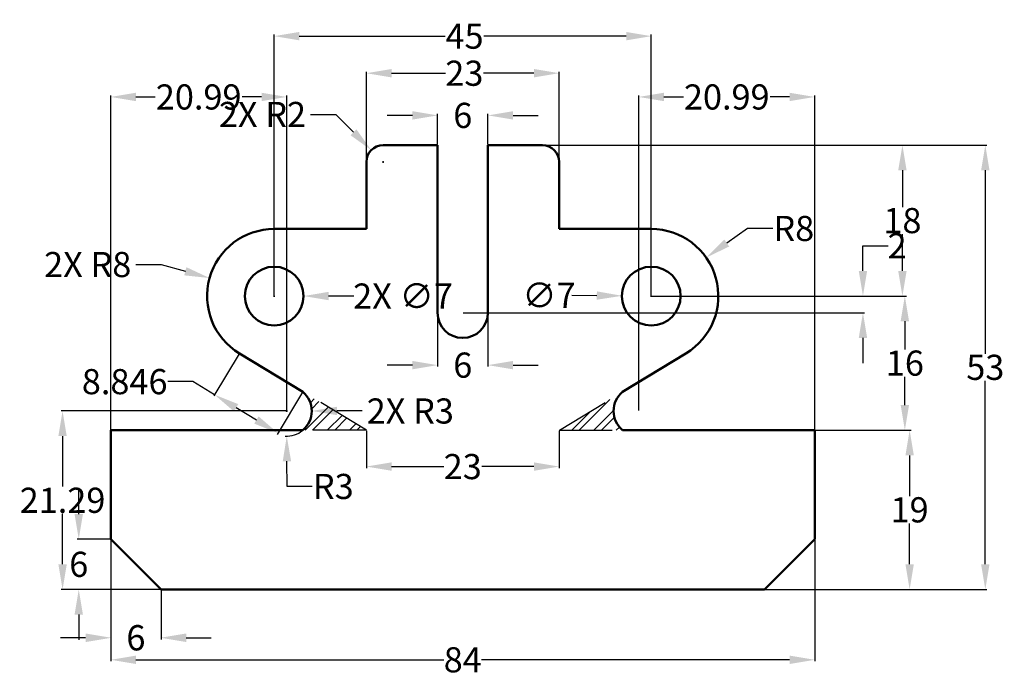
# Model space of a CAD drawing. Units: inches. Extents: x 2 to 120, y -4 to 75.
import ezdxf

# ---------------------------------------------------------------- set-up
doc = ezdxf.new("R2010")
doc.units = ezdxf.units.IN
doc.header["$MEASUREMENT"] = 0
doc.linetypes.add('HIDDEN', pattern=[9.525, 6.35, -3.175])
for name, color, linetype, lineweight in [('M-DIMS', 2, 'Continuous', 25), ('M-HATC', 8, 'Continuous', 18), ('M-HIDN', 8, 'HIDDEN', 25), ('M-OUTL', 7, 'Continuous', 50)]:
    doc.layers.add(name, color=color, linetype=linetype, lineweight=lineweight)
doc.styles.get("Standard").update_dxf_attribs({"font": 'arial.ttf'})
doc.dimstyles.get("Standard").update_dxf_attribs({"dimtxt": 3, "dimasz": 3, "dimexe": 0.18, "dimexo": 0.0625, "dimgap": 0.09, "dimtad": 0, "dimtih": 1, "dimtoh": 1, "dimdec": 4, "dimdsep": 46, "dimtxsty": 'Standard', "dimcen": 0.09, "dimadec": 0, "dimazin": 0, "dimtfac": 1, "dimtdec": 4, "dimtofl": 0, "dimtmove": 0, "dimatfit": 3, "dimfxl": 1, "dimtolj": 1, "dimtzin": 0, "dimarcsym": 0})

# ---------------------------------------------------------------- blocks, each defined once
blk = doc.blocks.new('*D1')
at = {"layer": 'Defpoints', "color": 0, "transparency": 16777216}
for p in [(43.51, 25.59), (66.51, 25.59), (66.51, 21.25)]:
    blk.add_point(p, dxfattribs=at)
at = {"layer": 'M-DIMS', "color": 0, "lineweight": -2, "transparency": 16777216}
for p, q in [((43.51, 25.53), (43.51, 21.07)), ((66.51, 25.53), (66.51, 21.07)), ((46.51, 21.25), (52.74, 21.25)), ((63.51, 21.25), (57.27, 21.25))]:
    blk.add_line(p, q, dxfattribs=at)
at = {"layer": 'M-DIMS', "color": 0, "transparency": 16777216}
for points in [[(46.51, 21.75), (46.51, 20.75), (43.51, 21.25)], [(63.51, 21.75), (63.51, 20.75), (66.51, 21.25)]]:
    blk.add_solid(points, dxfattribs=at)
at = {"layer": 'M-DIMS', "color": 0, "transparency": 16777216, "insert": (55.01, 21.25), "char_height": 3, "attachment_point": 5}
blk.add_mtext('\\A1;23', dxfattribs=at)
blk = doc.blocks.new('*D2')
at = {"layer": 'Defpoints', "color": 0, "transparency": 16777216}
for p in [(13.01, 12.59), (97.01, 12.59), (97.01, -1.8)]:
    blk.add_point(p, dxfattribs=at)
at = {"layer": 'M-DIMS', "color": 0, "lineweight": -2, "transparency": 16777216}
for p, q in [((13.01, 12.53), (13.01, -1.98)), ((97.01, 12.53), (97.01, -1.98)), ((16.01, -1.8), (52.77, -1.8)), ((94.01, -1.8), (57.24, -1.8))]:
    blk.add_line(p, q, dxfattribs=at)
at = {"layer": 'M-DIMS', "color": 0, "transparency": 16777216}
for points in [[(16.01, -1.3), (16.01, -2.3), (13.01, -1.8)], [(94.01, -1.3), (94.01, -2.3), (97.01, -1.8)]]:
    blk.add_solid(points, dxfattribs=at)
at = {"layer": 'M-DIMS', "color": 0, "transparency": 16777216, "insert": (55.01, -1.8), "char_height": 3, "attachment_point": 5}
blk.add_mtext('\\A1;84', dxfattribs=at)
blk = doc.blocks.new('*D3')
at = {"layer": 'Defpoints', "color": 0, "transparency": 16777216}
for p in [(13.01, 12.59), (9.19, 6.59), (19.01, 6.59)]:
    blk.add_point(p, dxfattribs=at)
at = {"layer": 'M-DIMS', "color": 0, "lineweight": -2, "transparency": 16777216}
for p, q in [((9.19, 15.59), (9.19, 18.59)), ((12.94, 12.59), (9.01, 12.59)), ((18.94, 6.59), (9.01, 6.59)), ((9.19, 3.59), (9.19, 0.59))]:
    blk.add_line(p, q, dxfattribs=at)
at = {"layer": 'M-DIMS', "color": 0, "transparency": 16777216}
for points in [[(8.69, 15.59), (9.69, 15.59), (9.19, 12.59)], [(8.69, 3.59), (9.69, 3.59), (9.19, 6.59)]]:
    blk.add_solid(points, dxfattribs=at)
at = {"layer": 'M-DIMS', "color": 0, "transparency": 16777216, "insert": (9.19, 9.59), "char_height": 3, "attachment_point": 5}
blk.add_mtext('\\A1;6', dxfattribs=at)
blk = doc.blocks.new('*D4')
at = {"layer": 'Defpoints', "color": 0, "transparency": 16777216}
for p in [(13.01, 12.59), (19.01, 6.59), (19.01, 0.82)]:
    blk.add_point(p, dxfattribs=at)
at = {"layer": 'M-DIMS', "color": 0, "lineweight": -2, "transparency": 16777216}
for p, q in [((13.01, 12.53), (13.01, 0.64)), ((19.01, 6.53), (19.01, 0.64)), ((10.01, 0.82), (7.01, 0.82)), ((22.01, 0.82), (25.01, 0.82))]:
    blk.add_line(p, q, dxfattribs=at)
at = {"layer": 'M-DIMS', "color": 0, "transparency": 16777216}
for points in [[(10.01, 1.32), (10.01, 0.32), (13.01, 0.82)], [(22.01, 1.32), (22.01, 0.32), (19.01, 0.82)]]:
    blk.add_solid(points, dxfattribs=at)
at = {"layer": 'M-DIMS', "color": 0, "transparency": 16777216, "insert": (16.01, 0.82), "char_height": 3, "attachment_point": 5}
blk.add_mtext('\\A1;6', dxfattribs=at)
blk = doc.blocks.new('*D5')
at = {"layer": 'Defpoints', "color": 0, "transparency": 16777216}
for p in [(52.01, 59.59), (58.01, 59.59), (58.01, 33.35)]:
    blk.add_point(p, dxfattribs=at)
at = {"layer": 'M-DIMS', "color": 0, "lineweight": -2, "transparency": 16777216}
for p, q in [((52.01, 59.53), (52.01, 33.17)), ((58.01, 59.53), (58.01, 33.17)), ((49.01, 33.35), (46.01, 33.35)), ((61.01, 33.35), (64.01, 33.35))]:
    blk.add_line(p, q, dxfattribs=at)
at = {"layer": 'M-DIMS', "color": 0, "transparency": 16777216}
for points in [[(49.01, 33.85), (49.01, 32.85), (52.01, 33.35)], [(61.01, 33.85), (61.01, 32.85), (58.01, 33.35)]]:
    blk.add_solid(points, dxfattribs=at)
at = {"layer": 'M-DIMS', "color": 0, "transparency": 16777216, "insert": (55.01, 33.35), "char_height": 3, "attachment_point": 5}
blk.add_mtext('\\A1;6', dxfattribs=at)
blk = doc.blocks.new('*D6')
at = {"layer": 'Defpoints', "color": 0, "transparency": 16777216}
for p in [(77.51, 72.59), (32.51, 41.59), (77.51, 41.59)]:
    blk.add_point(p, dxfattribs=at)
at = {"layer": 'M-DIMS', "color": 0, "lineweight": -2, "transparency": 16777216}
for p, q in [((32.51, 41.65), (32.51, 72.77)), ((35.51, 72.59), (52.91, 72.59)), ((74.51, 72.59), (57.53, 72.59)), ((77.51, 41.65), (77.51, 72.77))]:
    blk.add_line(p, q, dxfattribs=at)
at = {"layer": 'M-DIMS', "color": 0, "transparency": 16777216}
for points in [[(35.51, 73.09), (35.51, 72.09), (32.51, 72.59)], [(74.51, 73.09), (74.51, 72.09), (77.51, 72.59)]]:
    blk.add_solid(points, dxfattribs=at)
at = {"layer": 'M-DIMS', "color": 0, "transparency": 16777216, "insert": (55.22, 72.59), "char_height": 3, "attachment_point": 5}
blk.add_mtext('\\A1;45', dxfattribs=at)
blk = doc.blocks.new('*D7')
at = {"layer": 'Defpoints', "color": 0, "transparency": 16777216}
for p in [(97.01, 25.59), (108.33, 25.59), (91.01, 6.59)]:
    blk.add_point(p, dxfattribs=at)
at = {"layer": 'M-DIMS', "color": 0, "lineweight": -2, "transparency": 16777216}
for p, q in [((97.07, 25.59), (108.51, 25.59)), ((108.33, 22.59), (108.33, 17.71)), ((108.33, 9.59), (108.33, 14.47)), ((91.07, 6.59), (108.51, 6.59))]:
    blk.add_line(p, q, dxfattribs=at)
at = {"layer": 'M-DIMS', "color": 0, "transparency": 16777216}
for points in [[(107.83, 22.59), (108.83, 22.59), (108.33, 25.59)], [(107.83, 9.59), (108.83, 9.59), (108.33, 6.59)]]:
    blk.add_solid(points, dxfattribs=at)
at = {"layer": 'M-DIMS', "color": 0, "transparency": 16777216, "insert": (108.33, 16.09), "char_height": 3, "attachment_point": 5}
blk.add_mtext('\\A1;19', dxfattribs=at)
blk = doc.blocks.new('*D8')
at = {"layer": 'Defpoints', "color": 0, "transparency": 16777216}
for p in [(58.01, 63.14), (52.01, 59.59), (58.01, 59.59)]:
    blk.add_point(p, dxfattribs=at)
at = {"layer": 'M-DIMS', "color": 0, "lineweight": -2, "transparency": 16777216}
for p, q in [((49.01, 63.14), (46.01, 63.14)), ((52.01, 59.65), (52.01, 63.32)), ((58.01, 59.65), (58.01, 63.32)), ((61.01, 63.14), (64.01, 63.14))]:
    blk.add_line(p, q, dxfattribs=at)
at = {"layer": 'M-DIMS', "color": 0, "transparency": 16777216}
for points in [[(49.01, 63.64), (49.01, 62.64), (52.01, 63.14)], [(61.01, 63.64), (61.01, 62.64), (58.01, 63.14)]]:
    blk.add_solid(points, dxfattribs=at)
at = {"layer": 'M-DIMS', "color": 0, "transparency": 16777216, "insert": (55.01, 63.14), "char_height": 3, "attachment_point": 5}
blk.add_mtext('\\A1;6', dxfattribs=at)
blk = doc.blocks.new('*D9')
at = {"layer": 'Defpoints', "color": 0, "transparency": 16777216}
for p in [(77.51, 41.59), (97.01, 25.59), (107.76, 25.59)]:
    blk.add_point(p, dxfattribs=at)
at = {"layer": 'M-DIMS', "color": 0, "lineweight": -2, "transparency": 16777216}
for p, q in [((77.57, 41.59), (107.94, 41.59)), ((107.76, 38.59), (107.76, 35.21)), ((107.76, 28.59), (107.76, 31.97)), ((97.07, 25.59), (107.94, 25.59))]:
    blk.add_line(p, q, dxfattribs=at)
at = {"layer": 'M-DIMS', "color": 0, "transparency": 16777216}
for points in [[(107.26, 38.59), (108.26, 38.59), (107.76, 41.59)], [(107.26, 28.59), (108.26, 28.59), (107.76, 25.59)]]:
    blk.add_solid(points, dxfattribs=at)
at = {"layer": 'M-DIMS', "color": 0, "transparency": 16777216, "insert": (107.76, 33.59), "char_height": 3, "attachment_point": 5}
blk.add_mtext('\\A1;16', dxfattribs=at)
blk = doc.blocks.new('*D10')
at = {"layer": 'Defpoints', "color": 0, "transparency": 16777216}
for p in [(64.51, 59.59), (107.47, 59.59), (77.51, 41.59)]:
    blk.add_point(p, dxfattribs=at)
at = {"layer": 'M-DIMS', "color": 0, "lineweight": -2, "transparency": 16777216}
for p, q in [((64.57, 59.59), (107.65, 59.59)), ((107.47, 56.59), (107.47, 52.21)), ((107.47, 44.59), (107.47, 48.97)), ((77.57, 41.59), (107.65, 41.59))]:
    blk.add_line(p, q, dxfattribs=at)
at = {"layer": 'M-DIMS', "color": 0, "transparency": 16777216}
for points in [[(106.97, 56.59), (107.97, 56.59), (107.47, 59.59)], [(106.97, 44.59), (107.97, 44.59), (107.47, 41.59)]]:
    blk.add_solid(points, dxfattribs=at)
at = {"layer": 'M-DIMS', "color": 0, "transparency": 16777216, "insert": (107.47, 50.59), "char_height": 3, "attachment_point": 5}
blk.add_mtext('\\A1;18', dxfattribs=at)
blk = doc.blocks.new('*D11')
at = {"layer": 'Defpoints', "color": 0, "transparency": 16777216}
for p in [(61.26, 59.59), (61.26, 6.59), (117.36, 6.59)]:
    blk.add_point(p, dxfattribs=at)
at = {"layer": 'M-DIMS', "color": 0, "lineweight": -2, "transparency": 16777216}
for p, q in [((61.32, 59.59), (117.54, 59.59)), ((117.36, 56.59), (117.36, 34.71)), ((117.36, 9.59), (117.36, 31.47)), ((61.32, 6.59), (117.54, 6.59))]:
    blk.add_line(p, q, dxfattribs=at)
at = {"layer": 'M-DIMS', "color": 0, "transparency": 16777216}
for points in [[(116.86, 56.59), (117.86, 56.59), (117.36, 59.59)], [(116.86, 9.59), (117.86, 9.59), (117.36, 6.59)]]:
    blk.add_solid(points, dxfattribs=at)
at = {"layer": 'M-DIMS', "color": 0, "transparency": 16777216, "insert": (117.36, 33.09), "char_height": 3, "attachment_point": 5}
blk.add_mtext('\\A1;53', dxfattribs=at)
blk = doc.blocks.new('*D12')
at = {"layer": 'Defpoints', "color": 0, "transparency": 16777216}
for p in [(74.01, 41.62), (81.01, 41.56)]:
    blk.add_point(p, dxfattribs=at)
at = {"layer": 'M-DIMS', "color": 0, "lineweight": -2, "transparency": 16777216}
for p, q in [((68.01, 41.68), (71.01, 41.65)), ((77.42, 41.59), (77.6, 41.59)), ((77.51, 41.5), (77.51, 41.68))]:
    blk.add_line(p, q, dxfattribs=at)
at = {"layer": 'M-DIMS', "color": 0, "transparency": 16777216}
blk.add_solid([(71.01, 42.15), (71, 41.15), (74.01, 41.62)], dxfattribs=at)
at = {"layer": 'M-DIMS', "color": 0, "transparency": 16777216, "insert": (65.3, 41.68), "char_height": 3, "attachment_point": 5}
blk.add_mtext('\\A1;∅7', dxfattribs=at)
blk = doc.blocks.new('*D13')
at = {"layer": 'Defpoints', "color": 0, "transparency": 16777216}
for p in [(34, 27.88), (34.01, 24.88)]:
    blk.add_point(p, dxfattribs=at)
at = {"layer": 'M-DIMS', "color": 0, "lineweight": -2, "transparency": 16777216}
for p, q in [((33.91, 27.88), (34.09, 27.88)), ((34, 27.79), (34, 27.97)), ((34.05, 18.88), (34.03, 21.88)), ((37.05, 18.88), (34.05, 18.88))]:
    blk.add_line(p, q, dxfattribs=at)
blk.add_arc((34, 27.88), 3, 266.8832, 309.0905, dxfattribs=at)
at = {"layer": 'M-DIMS', "color": 0, "transparency": 16777216}
blk.add_solid([(34.53, 21.88), (33.53, 21.88), (34.01, 24.88)], dxfattribs=at)
at = {"layer": 'M-DIMS', "color": 0, "transparency": 16777216, "insert": (39.56, 18.88), "char_height": 3, "attachment_point": 5}
blk.add_mtext('\\A1;R3', dxfattribs=at)
blk = doc.blocks.new('*D14')
at = {"layer": 'Defpoints', "color": 0, "transparency": 16777216}
for p in [(84.06, 46.18), (77.51, 41.59)]:
    blk.add_point(p, dxfattribs=at)
at = {"layer": 'M-DIMS', "color": 0, "lineweight": -2, "transparency": 16777216}
for p, q in [((88.99, 49.65), (86.51, 47.91)), ((91.99, 49.65), (88.99, 49.65)), ((77.42, 41.59), (77.6, 41.59)), ((77.51, 41.5), (77.51, 41.68))]:
    blk.add_line(p, q, dxfattribs=at)
at = {"layer": 'M-DIMS', "color": 0, "transparency": 16777216}
blk.add_solid([(86.22, 48.32), (86.8, 47.5), (84.06, 46.18)], dxfattribs=at)
at = {"layer": 'M-DIMS', "color": 0, "transparency": 16777216, "insert": (94.51, 49.65), "char_height": 3, "attachment_point": 5}
blk.add_mtext('\\A1;R8', dxfattribs=at)
blk = doc.blocks.new('*D15')
at = {"layer": 'Defpoints', "color": 0, "transparency": 16777216}
for p in [(66.51, 68.17), (43.51, 53.59), (66.51, 53.59)]:
    blk.add_point(p, dxfattribs=at)
at = {"layer": 'M-DIMS', "color": 0, "lineweight": -2, "transparency": 16777216}
for p, q in [((43.51, 53.65), (43.51, 68.35)), ((46.51, 68.17), (52.94, 68.17)), ((63.51, 68.17), (57.47, 68.17)), ((66.51, 53.65), (66.51, 68.35))]:
    blk.add_line(p, q, dxfattribs=at)
at = {"layer": 'M-DIMS', "color": 0, "transparency": 16777216}
for points in [[(46.51, 68.67), (46.51, 67.67), (43.51, 68.17)], [(63.51, 68.67), (63.51, 67.67), (66.51, 68.17)]]:
    blk.add_solid(points, dxfattribs=at)
at = {"layer": 'M-DIMS', "color": 0, "transparency": 16777216, "insert": (55.2, 68.17), "char_height": 3, "attachment_point": 5}
blk.add_mtext('\\A1;23', dxfattribs=at)
blk = doc.blocks.new('*D16')
at = {"layer": 'Defpoints', "color": 0, "transparency": 16777216}
for p in [(13.005494, 12.589881), (19.005494, 6.589881), (19.005494, 0.839881)]:
    blk.add_point(p, dxfattribs=at)
at = {"layer": 'M-DIMS', "color": 0, "lineweight": -2, "transparency": 16777216}
for p, q in [((13.005494, 12.527381), (13.005494, 0.659881)), ((19.005494, 6.527381), (19.005494, 0.659881)), ((10.005494, 0.839881), (7.005494, 0.839881)), ((22.005494, 0.839881), (25.005494, 0.839881))]:
    blk.add_line(p, q, dxfattribs=at)
at = {"layer": 'M-DIMS', "color": 0, "transparency": 16777216}
for points in [[(10.005494, 1.339881), (10.005494, 0.339881), (13.005494, 0.839881)], [(22.005494, 1.339881), (22.005494, 0.339881), (19.005494, 0.839881)]]:
    blk.add_solid(points, dxfattribs=at)
at = {"layer": 'M-DIMS', "color": 0, "transparency": 16777216, "insert": (16.005494, 0.839881), "char_height": 3, "attachment_point": 5}
blk.add_mtext('\\A1;6', dxfattribs=at)
blk = doc.blocks.new('*D17')
at = {"layer": 'Defpoints', "color": 0, "transparency": 16777216}
for p in [(34, 65.34), (34, 27.88), (13.01, 25.59)]:
    blk.add_point(p, dxfattribs=at)
at = {"layer": 'M-DIMS', "color": 0, "lineweight": -2, "transparency": 16777216}
for p, q in [((13.01, 25.65), (13.01, 65.52)), ((16.01, 65.34), (18.32, 65.34)), ((31, 65.34), (28.68, 65.34)), ((34, 27.94), (34, 65.52))]:
    blk.add_line(p, q, dxfattribs=at)
at = {"layer": 'M-DIMS', "color": 0, "transparency": 16777216}
for points in [[(16.01, 65.84), (16.01, 64.84), (13.01, 65.34)], [(31, 65.84), (31, 64.84), (34, 65.34)]]:
    blk.add_solid(points, dxfattribs=at)
at = {"layer": 'M-DIMS', "color": 0, "transparency": 16777216, "insert": (23.5, 65.34), "char_height": 3, "attachment_point": 5}
blk.add_mtext('\\A1;20.99', dxfattribs=at)
blk = doc.blocks.new('*D18')
at = {"layer": 'Defpoints', "color": 0, "transparency": 16777216}
for p in [(76.01, 65.34), (76.01, 27.88), (97.01, 25.59)]:
    blk.add_point(p, dxfattribs=at)
at = {"layer": 'M-DIMS', "color": 0, "lineweight": -2, "transparency": 16777216}
for p, q in [((76.01, 27.94), (76.01, 65.52)), ((79.01, 65.34), (81.33, 65.34)), ((94.01, 65.34), (91.69, 65.34)), ((97.01, 25.65), (97.01, 65.52))]:
    blk.add_line(p, q, dxfattribs=at)
at = {"layer": 'M-DIMS', "color": 0, "transparency": 16777216}
for points in [[(79.01, 65.84), (79.01, 64.84), (76.01, 65.34)], [(94.01, 65.84), (94.01, 64.84), (97.01, 65.34)]]:
    blk.add_solid(points, dxfattribs=at)
at = {"layer": 'M-DIMS', "color": 0, "transparency": 16777216, "insert": (86.51, 65.34), "char_height": 3, "attachment_point": 5}
blk.add_mtext('\\A1;20.99', dxfattribs=at)
blk = doc.blocks.new('*D19')
at = {"layer": 'Defpoints', "color": 0, "transparency": 16777216}
for p in [(7.26, 27.88), (34, 27.88), (19.01, 6.59)]:
    blk.add_point(p, dxfattribs=at)
at = {"layer": 'M-DIMS', "color": 0, "lineweight": -2, "transparency": 16777216}
for p, q in [((33.93, 27.88), (7.08, 27.88)), ((7.26, 24.88), (7.26, 18.86)), ((7.26, 9.59), (7.26, 15.61)), ((18.94, 6.59), (7.08, 6.59))]:
    blk.add_line(p, q, dxfattribs=at)
at = {"layer": 'M-DIMS', "color": 0, "transparency": 16777216}
for points in [[(6.76, 24.88), (7.76, 24.88), (7.26, 27.88)], [(6.76, 9.59), (7.76, 9.59), (7.26, 6.59)]]:
    blk.add_solid(points, dxfattribs=at)
at = {"layer": 'M-DIMS', "color": 0, "transparency": 16777216, "insert": (7.26, 17.23), "char_height": 3, "attachment_point": 5}
blk.add_mtext('\\A1;21.29', dxfattribs=at)
blk = doc.blocks.new('*D20')
at = {"layer": 'Defpoints', "color": 0, "transparency": 16777216}
for p in [(28.37, 34.74), (25.39, 29.82), (35.94, 30.17)]:
    blk.add_point(p, dxfattribs=at)
at = {"layer": 'M-DIMS', "color": 0, "lineweight": -2, "transparency": 16777216}
for p, q in [((28.33, 34.69), (25.3, 29.67)), ((22.82, 31.38), (19.82, 31.38)), ((25.39, 29.82), (22.82, 31.38)), ((35.9, 30.11), (32.87, 25.09)), ((30.39, 26.8), (27.96, 28.27))]:
    blk.add_line(p, q, dxfattribs=at)
at = {"layer": 'M-DIMS', "color": 0, "transparency": 16777216}
for points in [[(28.22, 28.7), (27.7, 27.84), (25.39, 29.82)], [(30.65, 27.23), (30.13, 26.37), (32.96, 25.25)]]:
    blk.add_solid(points, dxfattribs=at)
at = {"layer": 'M-DIMS', "color": 0, "transparency": 16777216, "insert": (14.67, 31.38), "char_height": 3, "attachment_point": 5}
blk.add_mtext('\\A1;8.846', dxfattribs=at)
blk = doc.blocks.new('*D21')
at = {"layer": 'Defpoints', "color": 0, "transparency": 16777216}
for p in [(81.01, 41.59), (102.76, 41.59), (55.01, 39.59)]:
    blk.add_point(p, dxfattribs=at)
at = {"layer": 'M-DIMS', "color": 0, "lineweight": -2, "transparency": 16777216}
for p, q in [((102.76, 44.59), (102.76, 47.59)), ((102.76, 47.59), (105.76, 47.59)), ((81.07, 41.59), (102.94, 41.59)), ((55.07, 39.59), (102.94, 39.59)), ((102.76, 36.59), (102.76, 33.59))]:
    blk.add_line(p, q, dxfattribs=at)
at = {"layer": 'M-DIMS', "color": 0, "transparency": 16777216}
for points in [[(102.26, 44.59), (103.26, 44.59), (102.76, 41.59)], [(102.26, 36.59), (103.26, 36.59), (102.76, 39.59)]]:
    blk.add_solid(points, dxfattribs=at)
at = {"layer": 'M-DIMS', "color": 0, "transparency": 16777216, "insert": (106.84, 47.59), "char_height": 3, "attachment_point": 5}
blk.add_mtext('\\A1;2', dxfattribs=at)
blk = doc.blocks.new('*D22')
at = {"layer": 'Defpoints', "color": 0, "transparency": 16777216}
for p in [(44.09, 59), (45.51, 57.59)]:
    blk.add_point(p, dxfattribs=at)
at = {"layer": 'M-DIMS', "color": 0, "lineweight": -2, "transparency": 16777216}
for p, q in [((36.85, 63.25), (39.85, 63.25)), ((39.85, 63.25), (41.97, 61.12)), ((45.42, 57.59), (45.6, 57.59)), ((45.51, 57.5), (45.51, 57.68))]:
    blk.add_line(p, q, dxfattribs=at)
at = {"layer": 'M-DIMS', "color": 0, "transparency": 16777216}
blk.add_solid([(42.32, 61.48), (41.62, 60.77), (44.09, 59)], dxfattribs=at)
at = {"layer": 'M-DIMS', "color": 0, "transparency": 16777216, "insert": (31.11, 63.25), "char_height": 3, "attachment_point": 5}
blk.add_mtext('\\A1;2X R2', dxfattribs=at)
blk = doc.blocks.new('*D23')
at = {"layer": 'Defpoints', "color": 0, "transparency": 16777216}
for p in [(29.01, 41.59), (36.01, 41.59)]:
    blk.add_point(p, dxfattribs=at)
at = {"layer": 'M-DIMS', "color": 0, "lineweight": -2, "transparency": 16777216}
for p, q in [((32.42, 41.59), (32.6, 41.59)), ((32.51, 41.5), (32.51, 41.68)), ((42.01, 41.59), (39.01, 41.59))]:
    blk.add_line(p, q, dxfattribs=at)
at = {"layer": 'M-DIMS', "color": 0, "transparency": 16777216}
blk.add_solid([(39.01, 42.09), (39.01, 41.09), (36.01, 41.59)], dxfattribs=at)
at = {"layer": 'M-DIMS', "color": 0, "transparency": 16777216, "insert": (47.88, 41.59), "char_height": 3, "attachment_point": 5}
blk.add_mtext('\\A1;2X ∅7', dxfattribs=at)
blk = doc.blocks.new('*D24')
at = {"layer": 'Defpoints', "color": 0, "transparency": 16777216}
for p in [(24.8, 43.74), (32.51, 41.59)]:
    blk.add_point(p, dxfattribs=at)
at = {"layer": 'M-DIMS', "color": 0, "lineweight": -2, "transparency": 16777216}
for p, q in [((16.02, 45.35), (19.02, 45.35)), ((19.02, 45.35), (21.91, 44.54)), ((32.42, 41.59), (32.6, 41.59)), ((32.51, 41.5), (32.51, 41.68))]:
    blk.add_line(p, q, dxfattribs=at)
at = {"layer": 'M-DIMS', "color": 0, "transparency": 16777216}
blk.add_solid([(22.04, 45.03), (21.78, 44.06), (24.8, 43.74)], dxfattribs=at)
at = {"layer": 'M-DIMS', "color": 0, "transparency": 16777216, "insert": (10.26, 45.35), "char_height": 3, "attachment_point": 5}
blk.add_mtext('\\A1;2X R8', dxfattribs=at)
blk = doc.blocks.new('*D25')
at = {"layer": 'Defpoints', "color": 0, "transparency": 16777216}
for p in [(34, 27.88), (37, 27.88)]:
    blk.add_point(p, dxfattribs=at)
at = {"layer": 'M-DIMS', "color": 0, "lineweight": -2, "transparency": 16777216}
for p, q in [((33.91, 27.88), (34.09, 27.88)), ((34, 27.79), (34, 27.97)), ((43, 27.88), (40, 27.88))]:
    blk.add_line(p, q, dxfattribs=at)
at = {"layer": 'M-DIMS', "color": 0, "transparency": 16777216}
blk.add_solid([(40, 28.38), (40, 27.38), (37, 27.88)], dxfattribs=at)
at = {"layer": 'M-DIMS', "color": 0, "transparency": 16777216, "insert": (48.75, 27.88), "char_height": 3, "attachment_point": 5}
blk.add_mtext('\\A1;2X R3', dxfattribs=at)

msp = doc.modelspace()

# ---------------------------------------------------------------- hatches: boundary and pattern name
at = {"layer": 'M-HATC', "transparency": 33554559}
h = msp.add_hatch(dxfattribs=at)
h.set_pattern_fill('ANSI32', color=256, scale=5)
h.paths.add_polyline_path([(35.9358, 30.16696, -0.463292321), (35.9358, 25.58988), (43.50549, 25.58988)])
h.paths.add_polyline_path([(74.07519, 30.16696), (66.56603, 25.58988), (74.07519, 25.58988, -0.463292321)])

# ---------------------------------------------------------------- linework, layer by layer
at = {"layer": 'M-HIDN'}
for p, q in [((43.50549, 25.58988), (35.9358, 30.16696)), ((66.56603, 25.58988), (74.07519, 30.16696)), ((43.50549, 25.58988), (35.9358, 25.58988)), ((66.50549, 25.58988), (74.07519, 25.58988))]:
    msp.add_line(p, q, dxfattribs=at)
at = {"layer": 'M-OUTL'}
for p, q in [((45.50549, 59.58988), (52.00549, 59.58988)), ((52.00549, 39.58988), (52.00549, 59.58988)), ((58.00549, 39.58988), (58.00549, 59.58988)), ((58.00549, 59.58988), (64.50549, 59.58988)), ((43.50549, 49.58988), (43.50549, 57.58988)), ((66.50549, 49.58988), (66.50549, 57.58988)), ((32.50549, 49.58988), (43.50549, 49.58988)), ((77.50549, 49.58988), (66.50549, 49.58988)), ((35.9358, 30.16696), (28.3661, 34.74405)), ((74.07519, 30.16696), (81.64489, 34.74405)), ((13.00549, 25.58988), (13.00549, 12.58988)), ((13.00549, 25.58988), (35.9358, 25.58988)), ((74.07519, 25.58988), (97.00549, 25.58988)), ((97.00549, 12.58988), (97.00549, 25.58988)), ((13.00549, 12.58988), (19.00549, 6.58988)), ((91.00549, 6.58988), (97.00549, 12.58988)), ((19.00549, 6.58988), (91.00549, 6.58988))]:
    msp.add_line(p, q, dxfattribs=at)
for centre in [(32.50549, 41.58988), (77.50549, 41.58988)]:
    msp.add_circle(centre, 3.5, dxfattribs=at)
for centre, radius, start, end in [((45.50549, 57.58988), 2, 90, 180), ((64.50549, 57.58988), 2, 0, 90), ((32.50549, 41.58988), 8, 90, 238.8403748), ((77.50549, 41.58988), 8, 301.1596252, 90), ((55.00549, 39.58988), 3, 180, 0), ((33.99606, 27.87842), 3, 310.2841456, 49.7158544), ((76.01493, 27.87842), 3, 130.2841456, 229.7158544)]:
    msp.add_arc(centre, radius, start, end, dxfattribs=at)

# ---------------------------------------------------------------- dimensions: what is measured, and where the dimension line sits
at = {"layer": 'M-DIMS', "transparency": 33554559}
for base, p1, p2, picture, middle in [((77.50549, 72.58506), (32.50549, 41.58988), (77.50549, 41.58988), '*D6', (55.21576, 72.58506)), ((66.50549, 68.16792), (43.50549, 53.58988), (66.50549, 53.58988), '*D15', (55.20168, 68.16792))]:
    dim = msp.add_linear_dim(base=base, p1=p1, p2=p2, dimstyle='Standard', override={"dimclrd": 0, "dimclre": 0, "dimclrt": 0}, dxfattribs=at)
    dim.commit()
    dim.dimension.update_dxf_attribs({"geometry": picture, "text_midpoint": middle, "dimtype": 160})
for base, p1, p2, override, picture, middle in [((33.99606, 65.33988), (13.00549, 25.58988), (33.99606, 27.87842), {"dimdec": 2, "dimlfac": 1, "dimrnd": 0, "dimzin": 0, "dimdsep": 46, "dimlunit": 2}, '*D17', (23.50078, 65.33988)), ((76.01493, 65.33988), (97.00549, 25.58988), (76.01493, 27.87842), {"dimdec": 2, "dimlfac": 1, "dimrnd": 0, "dimzin": 0, "dimdsep": 46, "dimlunit": 2}, '*D18', (86.51021, 65.33988)), ((58.00549, 63.14138), (52.00549, 59.58988), (58.00549, 59.58988), {"dimclrd": 0, "dimclre": 0, "dimclrt": 0}, '*D8', (55.00549, 63.14138)), ((58.00549, 33.35332), (52.00549, 59.58988), (58.00549, 59.58988), {"dimclrd": 0, "dimclre": 0, "dimclrt": 0}, '*D5', (55.00549, 33.35332)), ((66.50549, 21.24957), (43.50549, 25.58988), (66.50549, 25.58988), {"dimclrd": 0, "dimclre": 0, "dimclrt": 0}, '*D1', (55.00549, 21.24957)), ((19.00549, 0.82102), (13.00549, 12.58988), (19.00549, 6.58988), {"dimclrd": 0, "dimclre": 0, "dimclrt": 0}, '*D4', (16.00549, 0.82102)), ((19.00549, 0.83988), (13.00549, 12.58988), (19.00549, 6.58988), {"dimdec": 0, "dimlfac": 1, "dimrnd": 0, "dimzin": 0, "dimdsep": 46, "dimlunit": 2}, '*D16', (16.00549, 0.83988)), ((97.00549, -1.79764), (13.00549, 12.58988), (97.00549, 12.58988), {"dimclrd": 0, "dimclre": 0, "dimclrt": 0}, '*D2', (55.00549, -1.79764))]:
    dim = msp.add_linear_dim(base=base, p1=p1, p2=p2, dimstyle='Standard', override=override, dxfattribs=at)
    dim.commit()
    dim.dimension.update_dxf_attribs({"geometry": picture, "text_midpoint": middle})
for center, mpoint, picture, middle in [((45.50549, 57.58988), (44.09109, 59.00391), '*D22', (31.10578, 63.24599)), ((32.50549, 41.58988), (24.79953, 43.73885), '*D24', (10.25952, 45.35058)), ((33.99606, 27.87842), (36.99606, 27.878), '*D25', (48.75352, 27.87716))]:
    dim = msp.add_radius_dim(center=center, mpoint=mpoint, text='2X <>', dimstyle='Standard', override={"dimdec": 0, "dimlfac": 1, "dimrnd": 0, "dimzin": 0, "dimdsep": 46, "dimlunit": 2}, dxfattribs=at)
    dim.commit()
    dim.dimension.update_dxf_attribs({"geometry": picture, "text_midpoint": middle})
for base, p1, p2, angle, override, picture, middle in [((117.35575, 6.58988), (61.25549, 59.58988), (61.25549, 6.58988), 90, {"dimclrd": 0, "dimclre": 0, "dimclrt": 0}, '*D11', (117.35575, 33.08988)), ((107.46666, 59.58988), (77.50549, 41.58988), (64.50549, 59.58988), 90, {"dimclrd": 0, "dimclre": 0, "dimclrt": 0}, '*D10', (107.46666, 50.58988)), ((102.75549, 41.58988), (55.00549, 39.58988), (81.00549, 41.58988), 90, {"dimdec": 0, "dimlfac": 1, "dimrnd": 0, "dimzin": 0, "dimdsep": 46, "dimlunit": 2}, '*D21', (106.83901, 47.58988)), ((107.75752, 25.58988), (77.50549, 41.58988), (97.00549, 25.58988), 90, {"dimclrd": 0, "dimclre": 0, "dimclrt": 0}, '*D9', (107.75752, 33.58988)), ((25.39091, 29.82361), (35.9358, 30.16696), (28.3661, 34.74405), 148.8403748, {"dimdec": 3, "dimlfac": 1, "dimrnd": 0, "dimzin": 0, "dimdsep": 46, "dimlunit": 2}, '*D20', (14.67097, 31.37588)), ((7.25549, 27.87842), (19.00549, 6.58988), (33.99606, 27.87842), 90, {"dimdec": 2, "dimlfac": 1, "dimrnd": 0, "dimzin": 0, "dimdsep": 46, "dimlunit": 2}, '*D19', (7.25549, 17.23415)), ((108.33203, 25.58988), (91.00549, 6.58988), (97.00549, 25.58988), 90, {"dimclrd": 0, "dimclre": 0, "dimclrt": 0}, '*D7', (108.33203, 16.08988)), ((9.18762, 6.58988), (13.00549, 12.58988), (19.00549, 6.58988), 90, {"dimclrd": 0, "dimclre": 0, "dimclrt": 0}, '*D3', (9.18762, 9.58988))]:
    dim = msp.add_linear_dim(base=base, p1=p1, p2=p2, angle=angle, dimstyle='Standard', override=override, dxfattribs=at)
    dim.commit()
    dim.dimension.update_dxf_attribs({"geometry": picture, "text_midpoint": middle})
dim = msp.add_radius_dim(center=(77.50549, 41.58988), mpoint=(84.0552, 46.18351), dimstyle='Standard', override={"dimclrd": 0, "dimclre": 0, "dimclrt": 0}, dxfattribs=at)
dim.commit()
dim.dimension.update_dxf_attribs({"geometry": '*D14', "text_midpoint": (94.50681, 49.64797), "dimtype": 164})
dim = msp.add_diameter_dim_2p(p1=(29.00549, 41.58976), p2=(36.00549, 41.59), text='2X <>', dimstyle='Standard', override={"dimdec": 0, "dimlfac": 1, "dimrnd": 0, "dimzin": 0, "dimdsep": 46, "dimlunit": 2}, dxfattribs=at)
dim.commit()
dim.dimension.update_dxf_attribs({"geometry": '*D23', "text_midpoint": (42.00549, 41.5902), "dimtype": 163})
dim = msp.add_diameter_dim_2p(p1=(81.00534, 41.5568), p2=(74.00565, 41.62296), dimstyle='Standard', override={"dimclrd": 0, "dimclre": 0, "dimclrt": 0}, dxfattribs=at)
dim.commit()
dim.dimension.update_dxf_attribs({"geometry": '*D12', "text_midpoint": (65.30064, 41.67967)})
dim = msp.add_radius_dim(center=(33.99606, 27.87842), mpoint=(34.01287, 24.87847), dimstyle='Standard', override={"dimclrd": 0, "dimclre": 0, "dimclrt": 0}, dxfattribs=at)
dim.commit()
dim.dimension.update_dxf_attribs({"geometry": '*D13', "text_midpoint": (39.5553, 18.87856)})

doc.saveas('drawing.dxf')
